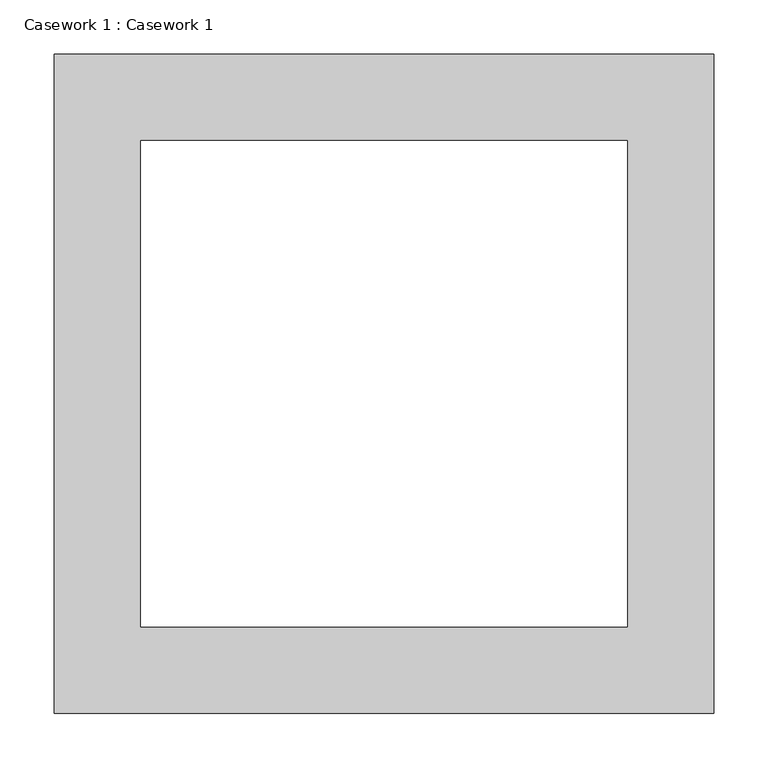
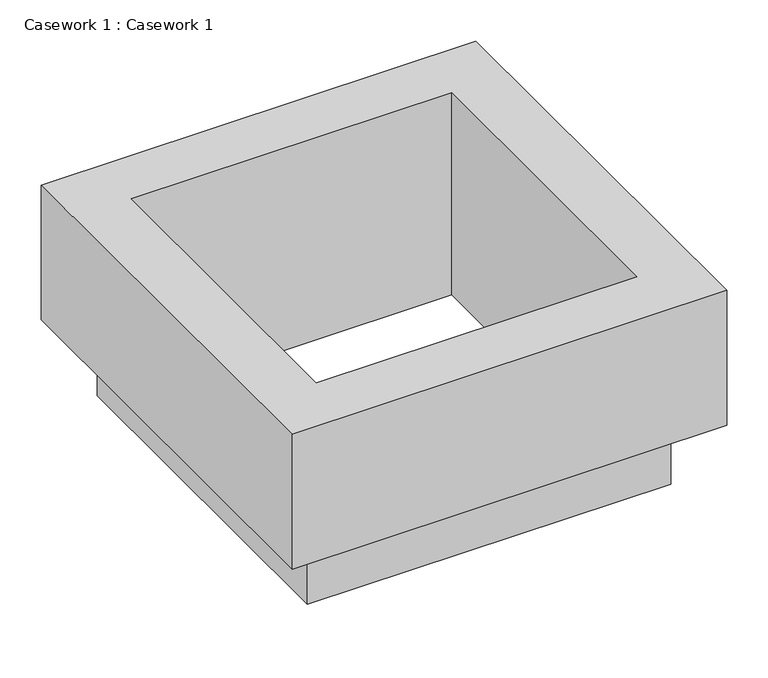
"""IFC4 building model written with IfcOpenShell, lengths in millimetres: furniture geometry, Casework 1 : Casework 1."""

from ifc_helpers import new_model, si_unit, origin, place, context, project, spatial, faceted_brep, source, transform, mapped, element, save


def casework_1_casework_1_62078cb6(model_context):
    return source(origin(), model_context, "Body", "Brep", [
        faceted_brep([(2918.0903786, -14053.8952964, 3550.0), (2918.0903786, -14053.8952964, 3450.0), (3428.0903786, -14053.8952964, 3450.0), (3428.0903786, -14053.8952964, 3550.0), (2868.0903786, -14103.8952964, 3750.0), (2868.0903786, -14103.8952964, 3550.0), (3478.0903786, -14103.8952964, 3550.0), (3478.0903786, -14103.8952964, 3750.0), (2948.0903786, -14023.8952964, 3450.0), (2948.0903786, -14023.8952964, 3750.0), (3398.0903786, -14023.8952964, 3750.0), (3398.0903786, -14023.8952964, 3450.0), (3428.0903786, -13543.8952964, 3450.0), (3428.0903786, -13543.8952964, 3550.0), (3478.0903786, -13493.8952964, 3550.0), (3478.0903786, -13493.8952964, 3750.0), (3398.0903786, -13573.8952964, 3750.0), (3398.0903786, -13573.8952964, 3450.0), (2918.0903786, -13543.8952964, 3450.0), (2918.0903786, -13543.8952964, 3550.0), (2868.0903786, -13493.8952964, 3550.0), (2868.0903786, -13493.8952964, 3750.0), (2948.0903786, -13573.8952964, 3750.0), (2948.0903786, -13573.8952964, 3450.0)], [[[0, 1, 2, 3]], [[4, 5, 6, 7]], [[8, 9, 10, 11]], [[3, 2, 12, 13]], [[7, 6, 14, 15]], [[11, 10, 16, 17]], [[13, 12, 18, 19]], [[15, 14, 20, 21]], [[17, 16, 22, 23]], [[19, 18, 1, 0]], [[5, 20, 14, 6], [3, 13, 19, 0]], [[21, 20, 5, 4]], [[7, 15, 21, 4], [9, 22, 16, 10]], [[23, 22, 9, 8]], [[1, 18, 12, 2], [11, 17, 23, 8]]]),
    ])


if __name__ == "__main__":
    model = new_model("IFC4")
    model_context = context("Model", 3, world=origin())
    ifc_project = project(units=[si_unit("LENGTHUNIT", "METRE", prefix="MILLI")], contexts=[model_context])
    site = spatial("IfcSite", under=ifc_project)
    building = spatial("IfcBuilding", under=site)
    placement = place(None, origin())
    casework_1_casework_1_shape = casework_1_casework_1_62078cb6(model_context)
    element("IfcFurniture", 1, ObjectType="Casework 1 : Casework 1", at=placement, inside=building, context=model_context, shape_type="MappedRepresentation", body=[
        mapped(casework_1_casework_1_shape, transform((0.0, 0.0, 0.0), x_axis=(1.0, 0.0, 0.0), y_axis=(0.0, 1.0, 0.0), z_axis=(0.0, 0.0, 1.0))),
    ])
    save(model, "model.ifc")
